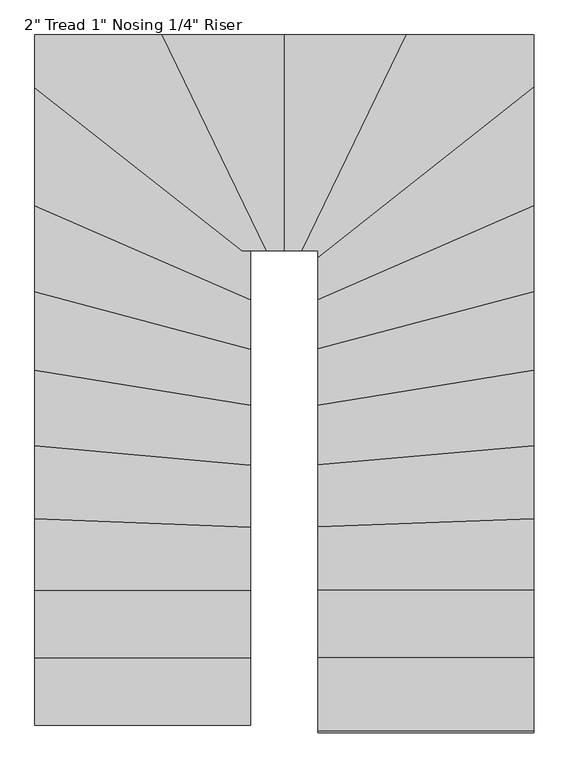
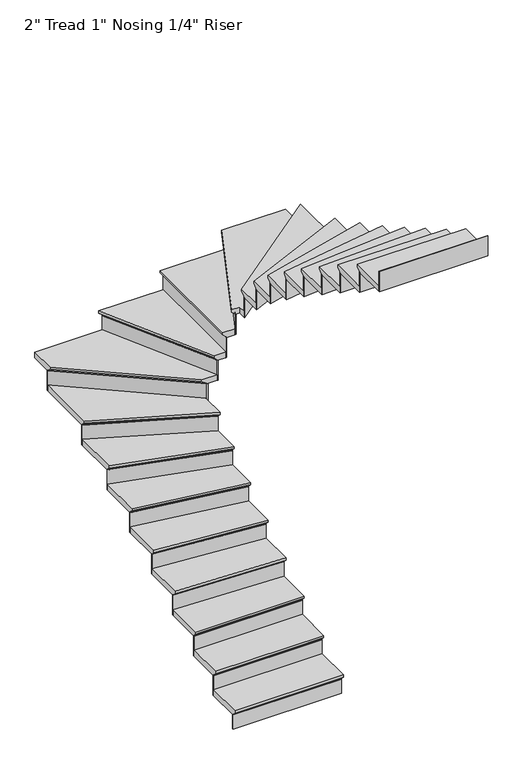
"""IFC4 building model written with IfcOpenShell, lengths in millimetres: stair flight geometry."""

from ifc_helpers import new_model, si_unit, origin, place, context, project, spatial, faceted_brep, source, transform, mapped, element, save


def stair_flight_c7d98fdd(model_context):
    return source(origin(), model_context, "Body", "Brep", [
        faceted_brep([(-5047.1987704, -4554.2130548, 47703.9214286), (-5047.1987704, -4554.2130548, 47722.9714286), (-5940.8822214, -4554.2130548, 47722.9714286), (-5940.8822214, -4554.2130548, 47703.9214286), (-5047.1987704, -4528.8130548, 47678.5214286), (-5940.8822214, -4528.8130548, 47678.5214286), (-5047.1987704, -4249.4130548, 47722.9714286), (-5940.8822214, -4249.4130548, 47722.9714286), (-5940.8822214, -4528.8130548, 47672.1714286), (-5940.8822214, -4249.4130548, 47672.1714286), (-5047.1987704, -4249.4130548, 47672.1714286), (-5047.1987704, -4528.8130548, 47672.1714286)], [[[0, 1, 2, 3]], [[4, 0, 3, 5]], [[2, 1, 6, 7]], [[8, 9, 10, 11]], [[2, 7, 9, 8, 5, 3]], [[8, 11, 4, 5]], [[6, 1, 0, 4, 11, 10]], [[7, 6, 10, 9]]]),
        faceted_brep([(-5047.1987704, -4528.8130548, 47672.1714286), (-5047.1987704, -4528.8130548, 47548.8), (-5047.1987704, -4522.4630548, 47548.8), (-5047.1987704, -4522.4630548, 47672.1714286), (-5940.8822214, -4528.8130548, 47672.1714286), (-5940.8822214, -4522.4630548, 47672.1714286), (-5940.8822214, -4522.4630548, 47548.8), (-5940.8822214, -4528.8130548, 47548.8)], [[[0, 1, 2, 3]], [[4, 5, 6, 7]], [[1, 0, 4, 7]], [[2, 1, 7, 6]], [[3, 2, 6, 5]], [[0, 3, 5, 4]]]),
        faceted_brep([(-5047.1987704, -4249.4130548, 47846.3428571), (-5047.1987704, -4249.4130548, 47672.1714286), (-5047.1987704, -4243.0630548, 47672.1714286), (-5047.1987704, -4243.0630548, 47846.3428571), (-5940.8822214, -4249.4130548, 47846.3428571), (-5940.8822214, -4243.0630548, 47846.3428571), (-5940.8822214, -4243.0630548, 47672.1714286), (-5940.8822214, -4249.4130548, 47672.1714286)], [[[0, 1, 2, 3]], [[4, 5, 6, 7]], [[1, 0, 4, 7]], [[2, 1, 7, 6]], [[3, 2, 6, 5]], [[0, 3, 5, 4]]]),
        faceted_brep([(-5940.8822214, -4274.8130548, 47897.1428571), (-5047.1987704, -4274.8130548, 47897.1428571), (-5047.1987704, -3970.0130548, 47897.1428571), (-5940.8822214, -3970.0130548, 47897.1428571), (-5940.8822214, -4249.4130548, 47846.3428571), (-5940.8822214, -3970.0130548, 47846.3428571), (-5047.1987704, -3970.0130548, 47846.3428571), (-5047.1987704, -4249.4130548, 47846.3428571), (-5940.8822214, -4249.4130548, 47852.6928571), (-5940.8822214, -4274.8130548, 47878.0928571), (-5047.1987704, -4249.4130548, 47852.6928571), (-5047.1987704, -4274.8130548, 47878.0928571)], [[[0, 1, 2, 3]], [[4, 5, 6, 7]], [[0, 3, 5, 4, 8, 9]], [[4, 7, 10, 8]], [[2, 1, 11, 10, 7, 6]], [[3, 2, 6, 5]], [[11, 1, 0, 9]], [[10, 11, 9, 8]]]),
        faceted_brep([(-5047.1987704, -3970.0130548, 48020.5142857), (-5047.1987704, -3970.0130548, 47846.3428571), (-5047.1987704, -3963.6630548, 47846.3428571), (-5047.1987704, -3963.6630548, 48020.5142857), (-5940.8822214, -3970.0130548, 48020.5142857), (-5940.8822214, -3963.6630548, 48020.5142857), (-5940.8822214, -3963.6630548, 47846.3428571), (-5940.8822214, -3970.0130548, 47846.3428571)], [[[0, 1, 2, 3]], [[4, 5, 6, 7]], [[1, 0, 4, 7]], [[2, 1, 7, 6]], [[3, 2, 6, 5]], [[0, 3, 5, 4]]]),
        faceted_brep([(-5940.8822214, -3995.4130548, 48071.3142857), (-5047.1987704, -3995.4130548, 48071.3142857), (-5047.1987704, -3707.9036879, 48071.3142857), (-5940.8822214, -3673.2843203, 48071.3142857), (-5940.8822214, -3970.0130548, 48020.5142857), (-5940.8822214, -3673.2843203, 48020.5142857), (-5047.1987704, -3707.9036879, 48020.5142857), (-5047.1987704, -3970.0130548, 48020.5142857), (-5940.8822214, -3970.0130548, 48026.8642857), (-5940.8822214, -3995.4130548, 48052.2642857), (-5047.1987704, -3970.0130548, 48026.8642857), (-5047.1987704, -3995.4130548, 48052.2642857)], [[[0, 1, 2, 3]], [[4, 5, 6, 7]], [[0, 3, 5, 4, 8, 9]], [[4, 7, 10, 8]], [[2, 1, 11, 10, 7, 6]], [[3, 2, 6, 5]], [[11, 1, 0, 9]], [[10, 11, 9, 8]]]),
        faceted_brep([(-5047.1987704, -3707.9036879, 48194.6857143), (-5047.1987704, -3707.9036879, 48020.5142857), (-5047.1987704, -3701.5489252, 48020.5142857), (-5047.1987704, -3701.5489252, 48194.6857143), (-5940.8822214, -3673.2843203, 48194.6857143), (-5940.8822214, -3666.9295576, 48194.6857143), (-5940.8822214, -3666.9295576, 48020.5142857), (-5940.8822214, -3673.2843203, 48020.5142857)], [[[0, 1, 2, 3]], [[4, 5, 6, 7]], [[1, 0, 4, 7]], [[2, 1, 7, 6]], [[3, 2, 6, 5]], [[0, 3, 5, 4]]]),
        faceted_brep([(-5940.8822214, -3698.703371, 48245.4857143), (-5047.1987704, -3733.3227386, 48245.4857143), (-5047.1987704, -3451.3234819, 48245.4857143), (-5940.8822214, -3370.89733, 48245.4857143), (-5940.8822214, -3673.2843203, 48194.6857143), (-5940.8822214, -3370.89733, 48194.6857143), (-5047.1987704, -3451.3234819, 48194.6857143), (-5047.1987704, -3707.9036879, 48194.6857143), (-5940.8822214, -3673.2843203, 48201.0357143), (-5940.8822214, -3698.703371, 48226.4357143), (-5047.1987704, -3707.9036879, 48201.0357143), (-5047.1987704, -3733.3227386, 48226.4357143)], [[[0, 1, 2, 3]], [[4, 5, 6, 7]], [[0, 3, 5, 4, 8, 9]], [[4, 7, 10, 8]], [[2, 1, 11, 10, 7, 6]], [[3, 2, 6, 5]], [[11, 1, 0, 9]], [[10, 11, 9, 8]]]),
        faceted_brep([(-5047.1987704, -3451.3234819, 48368.8571429), (-5047.1987704, -3451.3234819, 48194.6857143), (-5047.1987704, -3444.9478197, 48194.6857143), (-5047.1987704, -3444.9478197, 48368.8571429), (-5940.8822214, -3370.89733, 48368.8571429), (-5940.8822214, -3364.5216678, 48368.8571429), (-5940.8822214, -3364.5216678, 48194.6857143), (-5940.8822214, -3370.89733, 48194.6857143)], [[[0, 1, 2, 3]], [[4, 5, 6, 7]], [[1, 0, 4, 7]], [[2, 1, 7, 6]], [[3, 2, 6, 5]], [[0, 3, 5, 4]]]),
        faceted_brep([(-5940.8822214, -3396.3999789, 48419.6571429), (-5047.1987704, -3476.8261308, 48419.6571429), (-5047.1987704, -3203.4301079, 48419.6571429), (-5940.8822214, -3059.5417727, 48419.6571429), (-5940.8822214, -3370.89733, 48368.8571429), (-5940.8822214, -3059.5417727, 48368.8571429), (-5047.1987704, -3203.4301079, 48368.8571429), (-5047.1987704, -3451.3234819, 48368.8571429), (-5940.8822214, -3370.89733, 48375.2071429), (-5940.8822214, -3396.3999789, 48400.6071429), (-5047.1987704, -3451.3234819, 48375.2071429), (-5047.1987704, -3476.8261308, 48400.6071429)], [[[0, 1, 2, 3]], [[4, 5, 6, 7]], [[0, 3, 5, 4, 8, 9]], [[4, 7, 10, 8]], [[2, 1, 11, 10, 7, 6]], [[3, 2, 6, 5]], [[11, 1, 0, 9]], [[10, 11, 9, 8]]]),
        faceted_brep([(-5047.1987704, -3203.4301079, 48543.0285714), (-5047.1987704, -3203.4301079, 48368.8571429), (-5047.1987704, -3196.9983292, 48368.8571429), (-5047.1987704, -3196.9983292, 48543.0285714), (-5940.8822214, -3059.5417727, 48543.0285714), (-5940.8822214, -3053.109994, 48543.0285714), (-5940.8822214, -3053.109994, 48368.8571429), (-5940.8822214, -3059.5417727, 48368.8571429)], [[[0, 1, 2, 3]], [[4, 5, 6, 7]], [[1, 0, 4, 7]], [[2, 1, 7, 6]], [[3, 2, 6, 5]], [[0, 3, 5, 4]]]),
        faceted_brep([(-5940.8822214, -3085.2688872, 48593.8285714), (-5047.1987704, -3229.1572224, 48593.8285714), (-5047.1987704, -2970.3553609, 48593.8285714), (-5940.8822214, -2732.7052783, 48593.8285714), (-5940.8822214, -3059.5417727, 48543.0285714), (-5940.8822214, -2732.7052783, 48543.0285714), (-5047.1987704, -2970.3553609, 48543.0285714), (-5047.1987704, -3203.4301079, 48543.0285714), (-5940.8822214, -3059.5417727, 48549.3785714), (-5940.8822214, -3085.2688872, 48574.7785714), (-5047.1987704, -3203.4301079, 48549.3785714), (-5047.1987704, -3229.1572224, 48574.7785714)], [[[0, 1, 2, 3]], [[4, 5, 6, 7]], [[0, 3, 5, 4, 8, 9]], [[4, 7, 10, 8]], [[2, 1, 11, 10, 7, 6]], [[3, 2, 6, 5]], [[11, 1, 0, 9]], [[10, 11, 9, 8]]]),
        faceted_brep([(-5047.1987704, -2970.3553609, 48717.2), (-5047.1987704, -2970.3553609, 48543.0285714), (-5047.1987704, -2963.7846771, 48543.0285714), (-5047.1987704, -2963.7846771, 48717.2), (-5940.8822214, -2732.7052783, 48717.2), (-5940.8822214, -2726.1345945, 48717.2), (-5940.8822214, -2726.1345945, 48543.0285714), (-5940.8822214, -2732.7052783, 48543.0285714)], [[[0, 1, 2, 3]], [[4, 5, 6, 7]], [[1, 0, 4, 7]], [[2, 1, 7, 6]], [[3, 2, 6, 5]], [[0, 3, 5, 4]]]),
        faceted_brep([(-5940.8822214, -2758.9880136, 48768.0), (-5047.1987704, -2996.6380961, 48768.0), (-5047.1987704, -2765.8050203, 48768.0), (-5940.8822214, -2375.5896532, 48768.0), (-5940.8822214, -2732.7052783, 48717.2), (-5940.8822214, -2375.5896532, 48717.2), (-5047.1987704, -2765.8050203, 48717.2), (-5047.1987704, -2970.3553609, 48717.2), (-5940.8822214, -2732.7052783, 48723.55), (-5940.8822214, -2758.9880136, 48748.95), (-5047.1987704, -2970.3553609, 48723.55), (-5047.1987704, -2996.6380961, 48748.95)], [[[0, 1, 2, 3]], [[4, 5, 6, 7]], [[0, 3, 5, 4, 8, 9]], [[4, 7, 10, 8]], [[2, 1, 11, 10, 7, 6]], [[3, 2, 6, 5]], [[11, 1, 0, 9]], [[10, 11, 9, 8]]]),
        faceted_brep([(-5047.1987704, -2765.8050203, 48891.3714286), (-5047.1987704, -2765.8050203, 48717.2), (-5047.1987704, -2758.8760908, 48717.2), (-5047.1987704, -2758.8760908, 48891.3714286), (-5940.8822214, -2375.5896532, 48891.3714286), (-5940.8822214, -2368.6607237, 48891.3714286), (-5940.8822214, -2368.6607237, 48717.2), (-5940.8822214, -2375.5896532, 48717.2)], [[[0, 1, 2, 3]], [[4, 5, 6, 7]], [[1, 0, 4, 7]], [[2, 1, 7, 6]], [[3, 2, 6, 5]], [[0, 3, 5, 4]]]),
        faceted_brep([(-5940.8822214, -2403.3053713, 48942.1714286), (-5047.1987704, -2793.5207384, 48942.1714286), (-5047.1987704, -2590.8424524, 48942.1714286), (-5040.8038639, -2590.8424524, 48942.1714286), (-5940.8822214, -1882.1944717, 48942.1714286), (-5940.8822214, -2375.5896532, 48891.3714286), (-5940.8822214, -1882.1944717, 48891.3714286), (-5040.8038639, -2590.8424524, 48891.3714286), (-5047.1987704, -2590.8424524, 48891.3714286), (-5047.1987704, -2765.8050203, 48891.3714286), (-5940.8822214, -2375.5896532, 48897.7214286), (-5940.8822214, -2403.3053713, 48923.1214286), (-5047.1987704, -2765.8050203, 48897.7214286), (-5047.1987704, -2793.5207384, 48923.1214286)], [[[0, 1, 2, 3, 4]], [[5, 6, 7, 8, 9]], [[0, 4, 6, 5, 10, 11]], [[5, 9, 12, 10]], [[2, 1, 13, 12, 9, 8]], [[4, 3, 7, 6]], [[13, 1, 0, 11]], [[12, 13, 11, 10]], [[3, 2, 8, 7]]]),
        faceted_brep([(-5040.8038639, -2590.8424524, 49065.5428571), (-5040.8038639, -2590.8424524, 48891.3714286), (-5030.5387554, -2590.8424524, 48891.3714286), (-5030.5387554, -2590.8424524, 49065.5428571), (-5940.8822214, -1882.1944717, 49065.5428571), (-5940.8822214, -1874.1125661, 49065.5428571), (-5940.8822214, -1874.1125661, 48891.3714286), (-5940.8822214, -1882.1944717, 48891.3714286)], [[[0, 1, 2, 3]], [[4, 5, 6, 7]], [[1, 0, 4, 7]], [[2, 1, 7, 6]], [[3, 2, 6, 5]], [[0, 3, 5, 4]]]),
        faceted_brep([(-5384.6489457, -1697.1590014, 49116.3428571), (-5940.8822214, -1697.1590014, 49116.3428571), (-5940.8822214, -1914.5220945, 49116.3428571), (-5081.8642978, -2590.8424524, 49116.3428571), (-4952.3566185, -2590.8424524, 49116.3428571), (-5940.8822214, -1697.1590014, 49065.5428571), (-5384.6489457, -1697.1590014, 49065.5428571), (-4952.3566185, -2590.8424524, 49065.5428571), (-5040.8038639, -2590.8424524, 49065.5428571), (-5940.8822214, -1882.1944717, 49065.5428571), (-5940.8822214, -1882.1944717, 49071.8928571), (-5940.8822214, -1914.5220945, 49097.2928571), (-5040.8038639, -2590.8424524, 49071.8928571), (-5081.8642978, -2590.8424524, 49097.2928571)], [[[0, 1, 2, 3, 4]], [[5, 6, 7, 8, 9]], [[1, 0, 6, 5]], [[2, 1, 5, 9, 10, 11]], [[9, 8, 12, 10]], [[4, 3, 13, 12, 8, 7]], [[0, 4, 7, 6]], [[13, 3, 2, 11]], [[12, 13, 11, 10]]]),
        faceted_brep([(-4952.3566185, -2590.8424524, 49239.7142857), (-4952.3566185, -2590.8424524, 49065.5428571), (-4945.3027294, -2590.8424524, 49065.5428571), (-4945.3027294, -2590.8424524, 49239.7142857), (-5384.6489457, -1697.1590014, 49239.7142857), (-5377.5950566, -1697.1590014, 49239.7142857), (-5377.5950566, -1697.1590014, 49065.5428571), (-5384.6489457, -1697.1590014, 49065.5428571)], [[[0, 1, 2, 3]], [[4, 5, 6, 7]], [[1, 0, 4, 7]], [[2, 1, 7, 6]], [[3, 2, 6, 5]], [[0, 3, 5, 4]]]),
        faceted_brep([(-5412.8645022, -1697.1590014, 49290.5142857), (-4980.5721749, -2590.8424524, 49290.5142857), (-4882.0987704, -2590.8424524, 49290.5142857), (-4882.0987706, -1697.1590014, 49290.5142857), (-5384.6489457, -1697.1590014, 49239.7142857), (-4882.0987706, -1697.1590014, 49239.7142857), (-4882.0987704, -2590.8424524, 49239.7142857), (-4952.3566185, -2590.8424524, 49239.7142857), (-5384.6489457, -1697.1590014, 49246.0642857), (-5412.8645022, -1697.1590014, 49271.4642857), (-4952.3566185, -2590.8424524, 49246.0642857), (-4980.5721749, -2590.8424524, 49271.4642857)], [[[0, 1, 2, 3]], [[4, 5, 6, 7]], [[0, 3, 5, 4, 8, 9]], [[4, 7, 10, 8]], [[3, 2, 6, 5]], [[11, 1, 0, 9]], [[10, 11, 9, 8]], [[2, 1, 11, 10, 7, 6]]]),
        faceted_brep([(-4882.0987704, -2590.8424524, 49413.8857143), (-4882.0987704, -2590.8424524, 49239.7142857), (-4875.7487704, -2590.8424524, 49239.7142857), (-4875.7487704, -2590.8424524, 49413.8857143), (-4882.0987706, -1697.1590014, 49413.8857143), (-4875.7487706, -1697.1590014, 49413.8857143), (-4875.7487706, -1697.1590014, 49239.7142857), (-4882.0987706, -1697.1590014, 49239.7142857)], [[[0, 1, 2, 3]], [[4, 5, 6, 7]], [[1, 0, 4, 7]], [[2, 1, 7, 6]], [[3, 2, 6, 5]], [[0, 3, 5, 4]]]),
        faceted_brep([(-4907.4987706, -1697.1590014, 49464.6857143), (-4907.4987704, -2590.8424524, 49464.6857143), (-4806.2098095, -2590.8424524, 49464.6857143), (-4373.9174828, -1697.1590014, 49464.6857143), (-4882.0987706, -1697.1590014, 49413.8857143), (-4373.9174828, -1697.1590014, 49413.8857143), (-4806.2098095, -2590.8424524, 49413.8857143), (-4882.0987704, -2590.8424524, 49413.8857143), (-4882.0987706, -1697.1590014, 49420.2357143), (-4907.4987706, -1697.1590014, 49445.6357143), (-4882.0987704, -2590.8424524, 49420.2357143), (-4907.4987704, -2590.8424524, 49445.6357143)], [[[0, 1, 2, 3]], [[4, 5, 6, 7]], [[0, 3, 5, 4, 8, 9]], [[4, 7, 10, 8]], [[2, 1, 11, 10, 7, 6]], [[3, 2, 6, 5]], [[11, 1, 0, 9]], [[10, 11, 9, 8]]]),
        faceted_brep([(-4806.2098095, -2590.8424524, 49588.0571429), (-4806.2098095, -2590.8424524, 49413.8857143), (-4799.1559204, -2590.8424524, 49413.8857143), (-4799.1559204, -2590.8424524, 49588.0571429), (-4373.9174828, -1697.1590014, 49588.0571429), (-4366.8635937, -1697.1590014, 49588.0571429), (-4366.8635937, -1697.1590014, 49413.8857143), (-4373.9174828, -1697.1590014, 49413.8857143)], [[[0, 1, 2, 3]], [[4, 5, 6, 7]], [[1, 0, 4, 7]], [[2, 1, 7, 6]], [[3, 2, 6, 5]], [[0, 3, 5, 4]]]),
        faceted_brep([(-3874.1153195, -1946.8497166, 49638.8571429), (-3874.1153195, -1697.1590014, 49638.8571429), (-4402.1330392, -1697.1590014, 49638.8571429), (-4834.4253659, -2590.8424524, 49638.8571429), (-4767.7987704, -2590.8424524, 49638.8571429), (-4767.7987704, -2650.4628721, 49638.8571429), (-3874.1153195, -1697.1590014, 49588.0571429), (-3874.1153195, -1946.8497166, 49588.0571429), (-4767.7987704, -2650.4628721, 49588.0571429), (-4767.7987704, -2590.8424524, 49588.0571429), (-4806.2098095, -2590.8424524, 49588.0571429), (-4373.9174828, -1697.1590014, 49588.0571429), (-4806.2098095, -2590.8424524, 49594.4071429), (-4373.9174828, -1697.1590014, 49594.4071429), (-4834.4253659, -2590.8424524, 49619.8071429), (-4402.1330392, -1697.1590014, 49619.8071429)], [[[0, 1, 2, 3, 4, 5]], [[6, 7, 8, 9, 10, 11]], [[1, 0, 7, 6]], [[11, 10, 12, 13]], [[4, 3, 14, 12, 10, 9]], [[5, 4, 9, 8]], [[0, 5, 8, 7]], [[14, 3, 2, 15]], [[12, 14, 15, 13]], [[2, 1, 6, 11, 13, 15]]]),
        faceted_brep([(-4767.7987704, -2650.4628721, 49762.2285714), (-4767.7987704, -2650.4628721, 49588.0571429), (-4767.7987704, -2658.5447778, 49588.0571429), (-4767.7987704, -2658.5447778, 49762.2285714), (-3874.1153195, -1946.8497166, 49762.2285714), (-3874.1153195, -1954.9316222, 49762.2285714), (-3874.1153195, -1954.9316222, 49588.0571429), (-3874.1153195, -1946.8497166, 49588.0571429)], [[[0, 1, 2, 3]], [[4, 5, 6, 7]], [[1, 0, 4, 7]], [[2, 1, 7, 6]], [[3, 2, 6, 5]], [[0, 3, 5, 4]]]),
        faceted_brep([(-3874.1153195, -1914.5220938, 49813.0285714), (-4767.7987704, -2618.1352494, 49813.0285714), (-4767.7987704, -2821.2364563, 49813.0285714), (-3874.1153195, -2431.0210889, 49813.0285714), (-3874.1153195, -1946.8497166, 49762.2285714), (-3874.1153195, -2431.0210889, 49762.2285714), (-4767.7987704, -2821.2364563, 49762.2285714), (-4767.7987704, -2650.4628721, 49762.2285714), (-3874.1153195, -1946.8497166, 49768.5785714), (-3874.1153195, -1914.5220938, 49793.9785714), (-4767.7987704, -2650.4628721, 49768.5785714), (-4767.7987704, -2618.1352494, 49793.9785714)], [[[0, 1, 2, 3]], [[4, 5, 6, 7]], [[0, 3, 5, 4, 8, 9]], [[4, 7, 10, 8]], [[2, 1, 11, 10, 7, 6]], [[3, 2, 6, 5]], [[11, 1, 0, 9]], [[10, 11, 9, 8]]]),
        faceted_brep([(-4767.7987704, -2821.2364563, 49936.4), (-4767.7987704, -2821.2364563, 49762.2285714), (-4767.7987704, -2828.1653858, 49762.2285714), (-4767.7987704, -2828.1653858, 49936.4), (-3874.1153195, -2431.0210889, 49936.4), (-3874.1153195, -2437.9500185, 49936.4), (-3874.1153195, -2437.9500185, 49762.2285714), (-3874.1153195, -2431.0210889, 49762.2285714)], [[[0, 1, 2, 3]], [[4, 5, 6, 7]], [[1, 0, 4, 7]], [[2, 1, 7, 6]], [[3, 2, 6, 5]], [[0, 3, 5, 4]]]),
        faceted_brep([(-3874.1153195, -2403.3053709, 49987.2), (-4767.7987704, -2793.5207382, 49987.2), (-4767.7987704, -3022.9208311, 49987.2), (-3874.1153195, -2785.2707484, 49987.2), (-3874.1153195, -2431.0210889, 49936.4), (-3874.1153195, -2785.2707484, 49936.4), (-4767.7987704, -3022.9208311, 49936.4), (-4767.7987704, -2821.2364563, 49936.4), (-3874.1153195, -2431.0210889, 49942.75), (-3874.1153195, -2403.3053709, 49968.15), (-4767.7987704, -2821.2364563, 49942.75), (-4767.7987704, -2793.5207382, 49968.15)], [[[0, 1, 2, 3]], [[4, 5, 6, 7]], [[0, 3, 5, 4, 8, 9]], [[4, 7, 10, 8]], [[2, 1, 11, 10, 7, 6]], [[3, 2, 6, 5]], [[11, 1, 0, 9]], [[10, 11, 9, 8]]]),
        faceted_brep([(-4767.7987704, -3022.9208311, 50110.5714286), (-4767.7987704, -3022.9208311, 49936.4), (-4767.7987704, -3029.4915149, 49936.4), (-4767.7987704, -3029.4915149, 50110.5714286), (-3874.1153195, -2785.2707484, 50110.5714286), (-3874.1153195, -2791.8414322, 50110.5714286), (-3874.1153195, -2791.8414322, 49936.4), (-3874.1153195, -2785.2707484, 49936.4)], [[[0, 1, 2, 3]], [[4, 5, 6, 7]], [[1, 0, 4, 7]], [[2, 1, 7, 6]], [[3, 2, 6, 5]], [[0, 3, 5, 4]]]),
        faceted_brep([(-3874.1153195, -2758.9880132, 50161.3714286), (-4767.7987704, -2996.6380959, 50161.3714286), (-4767.7987704, -3254.8843368, 50161.3714286), (-3874.1153195, -3110.9960015, 50161.3714286), (-3874.1153195, -2785.2707484, 50110.5714286), (-3874.1153195, -3110.9960015, 50110.5714286), (-4767.7987704, -3254.8843368, 50110.5714286), (-4767.7987704, -3022.9208311, 50110.5714286), (-3874.1153195, -2785.2707484, 50116.9214286), (-3874.1153195, -2758.9880132, 50142.3214286), (-4767.7987704, -3022.9208311, 50116.9214286), (-4767.7987704, -2996.6380959, 50142.3214286)], [[[0, 1, 2, 3]], [[4, 5, 6, 7]], [[0, 3, 5, 4, 8, 9]], [[4, 7, 10, 8]], [[2, 1, 11, 10, 7, 6]], [[3, 2, 6, 5]], [[11, 1, 0, 9]], [[10, 11, 9, 8]]]),
        faceted_brep([(-4767.7987704, -3254.8843368, 50284.7428571), (-4767.7987704, -3254.8843368, 50110.5714286), (-4767.7987704, -3261.3161154, 50110.5714286), (-4767.7987704, -3261.3161154, 50284.7428571), (-3874.1153195, -3110.9960015, 50284.7428571), (-3874.1153195, -3117.4277801, 50284.7428571), (-3874.1153195, -3117.4277801, 50110.5714286), (-3874.1153195, -3110.9960015, 50110.5714286)], [[[0, 1, 2, 3]], [[4, 5, 6, 7]], [[1, 0, 4, 7]], [[2, 1, 7, 6]], [[3, 2, 6, 5]], [[0, 3, 5, 4]]]),
        faceted_brep([(-3874.1153195, -3085.2688869, 50335.5428571), (-4767.7987704, -3229.1572222, 50335.5428571), (-4767.7987704, -3502.3287795, 50335.5428571), (-3874.1153195, -3421.9026274, 50335.5428571), (-3874.1153195, -3110.9960015, 50284.7428571), (-3874.1153195, -3421.9026274, 50284.7428571), (-4767.7987704, -3502.3287795, 50284.7428571), (-4767.7987704, -3254.8843368, 50284.7428571), (-3874.1153195, -3110.9960015, 50291.0928571), (-3874.1153195, -3085.2688869, 50316.4928571), (-4767.7987704, -3254.8843368, 50291.0928571), (-4767.7987704, -3229.1572222, 50316.4928571)], [[[0, 1, 2, 3]], [[4, 5, 6, 7]], [[0, 3, 5, 4, 8, 9]], [[4, 7, 10, 8]], [[2, 1, 11, 10, 7, 6]], [[3, 2, 6, 5]], [[11, 1, 0, 9]], [[10, 11, 9, 8]]]),
        faceted_brep([(-4767.7987704, -3502.3287795, 50458.9142857), (-4767.7987704, -3502.3287795, 50284.7428571), (-4767.7987704, -3508.7044417, 50284.7428571), (-4767.7987704, -3508.7044417, 50458.9142857), (-3874.1153195, -3421.9026274, 50458.9142857), (-3874.1153195, -3428.2782897, 50458.9142857), (-3874.1153195, -3428.2782897, 50284.7428571), (-3874.1153195, -3421.9026274, 50284.7428571)], [[[0, 1, 2, 3]], [[4, 5, 6, 7]], [[1, 0, 4, 7]], [[2, 1, 7, 6]], [[3, 2, 6, 5]], [[0, 3, 5, 4]]]),
        faceted_brep([(-3874.1153195, -3396.3999786, 50509.7142857), (-4767.7987704, -3476.8261306, 50509.7142857), (-4767.7987704, -3758.7417891, 50509.7142857), (-3874.1153195, -3724.1224215, 50509.7142857), (-3874.1153195, -3421.9026274, 50458.9142857), (-3874.1153195, -3724.1224215, 50458.9142857), (-4767.7987704, -3758.7417891, 50458.9142857), (-4767.7987704, -3502.3287795, 50458.9142857), (-3874.1153195, -3421.9026274, 50465.2642857), (-3874.1153195, -3396.3999786, 50490.6642857), (-4767.7987704, -3502.3287795, 50465.2642857), (-4767.7987704, -3476.8261306, 50490.6642857)], [[[0, 1, 2, 3]], [[4, 5, 6, 7]], [[0, 3, 5, 4, 8, 9]], [[4, 7, 10, 8]], [[2, 1, 11, 10, 7, 6]], [[3, 2, 6, 5]], [[11, 1, 0, 9]], [[10, 11, 9, 8]]]),
        faceted_brep([(-4767.7987704, -3758.7417891, 50633.0857143), (-4767.7987704, -3758.7417891, 50458.9142857), (-4767.7987704, -3765.0965518, 50458.9142857), (-4767.7987704, -3765.0965518, 50633.0857143), (-3874.1153195, -3724.1224215, 50633.0857143), (-3874.1153195, -3730.4771842, 50633.0857143), (-3874.1153195, -3730.4771842, 50458.9142857), (-3874.1153195, -3724.1224215, 50458.9142857)], [[[0, 1, 2, 3]], [[4, 5, 6, 7]], [[1, 0, 4, 7]], [[2, 1, 7, 6]], [[3, 2, 6, 5]], [[0, 3, 5, 4]]]),
        faceted_brep([(-3874.1153195, -3698.7033708, 50683.8857143), (-4767.7987704, -3733.3227384, 50683.8857143), (-4767.7987704, -4020.8130546, 50683.8857143), (-3874.1153195, -4020.8130546, 50683.8857143), (-3874.1153195, -3724.1224215, 50633.0857143), (-3874.1153195, -4020.8130546, 50633.0857143), (-4767.7987704, -4020.8130546, 50633.0857143), (-4767.7987704, -3758.7417891, 50633.0857143), (-3874.1153195, -3724.1224215, 50639.4357143), (-3874.1153195, -3698.7033708, 50664.8357143), (-4767.7987704, -3758.7417891, 50639.4357143), (-4767.7987704, -3733.3227384, 50664.8357143)], [[[0, 1, 2, 3]], [[4, 5, 6, 7]], [[0, 3, 5, 4, 8, 9]], [[4, 7, 10, 8]], [[2, 1, 11, 10, 7, 6]], [[3, 2, 6, 5]], [[11, 1, 0, 9]], [[10, 11, 9, 8]]]),
        faceted_brep([(-4767.7987704, -4020.8130546, 50807.2571429), (-4767.7987704, -4020.8130546, 50633.0857143), (-4767.7987704, -4027.1630546, 50633.0857143), (-4767.7987704, -4027.1630546, 50807.2571429), (-3874.1153195, -4020.8130546, 50807.2571429), (-3874.1153195, -4027.1630546, 50807.2571429), (-3874.1153195, -4027.1630546, 50633.0857143), (-3874.1153195, -4020.8130546, 50633.0857143)], [[[0, 1, 2, 3]], [[4, 5, 6, 7]], [[1, 0, 4, 7]], [[2, 1, 7, 6]], [[3, 2, 6, 5]], [[0, 3, 5, 4]]]),
        faceted_brep([(-3874.1153195, -3995.4130546, 50858.0571429), (-4767.7987704, -3995.4130546, 50858.0571429), (-4767.7987704, -4300.2130546, 50858.0571429), (-3874.1153195, -4300.2130546, 50858.0571429), (-3874.1153195, -4020.8130546, 50807.2571429), (-3874.1153195, -4300.2130546, 50807.2571429), (-4767.7987704, -4300.2130546, 50807.2571429), (-4767.7987704, -4020.8130546, 50807.2571429), (-3874.1153195, -4020.8130546, 50813.6071429), (-3874.1153195, -3995.4130546, 50839.0071429), (-4767.7987704, -4020.8130546, 50813.6071429), (-4767.7987704, -3995.4130546, 50839.0071429)], [[[0, 1, 2, 3]], [[4, 5, 6, 7]], [[0, 3, 5, 4, 8, 9]], [[4, 7, 10, 8]], [[2, 1, 11, 10, 7, 6]], [[3, 2, 6, 5]], [[11, 1, 0, 9]], [[10, 11, 9, 8]]]),
        faceted_brep([(-4767.7987704, -4300.2130546, 50981.4285714), (-4767.7987704, -4300.2130546, 50807.2571429), (-4767.7987704, -4306.5630546, 50807.2571429), (-4767.7987704, -4306.5630546, 50981.4285714), (-3874.1153195, -4300.2130546, 50981.4285714), (-3874.1153195, -4306.5630546, 50981.4285714), (-3874.1153195, -4306.5630546, 50807.2571429), (-3874.1153195, -4300.2130546, 50807.2571429)], [[[0, 1, 2, 3]], [[4, 5, 6, 7]], [[1, 0, 4, 7]], [[2, 1, 7, 6]], [[3, 2, 6, 5]], [[0, 3, 5, 4]]]),
        faceted_brep([(-4767.7987704, -4579.6130546, 51155.6), (-4767.7987704, -4579.6130546, 50981.4285714), (-4767.7987704, -4585.9630546, 50981.4285714), (-4767.7987704, -4585.9630546, 51155.6), (-3874.1153195, -4579.6130546, 51155.6), (-3874.1153195, -4585.9630546, 51155.6), (-3874.1153195, -4585.9630546, 50981.4285714), (-3874.1153195, -4579.6130546, 50981.4285714)], [[[0, 1, 2, 3]], [[4, 5, 6, 7]], [[1, 0, 4, 7]], [[2, 1, 7, 6]], [[3, 2, 6, 5]], [[0, 3, 5, 4]]]),
        faceted_brep([(-3874.1153195, -4274.8130546, 51032.2285714), (-4767.7987704, -4274.8130546, 51032.2285714), (-4767.7987704, -4579.6130546, 51032.2285714), (-3874.1153195, -4579.6130546, 51032.2285714), (-3874.1153195, -4300.2130546, 50981.4285714), (-3874.1153195, -4579.6130546, 50981.4285714), (-4767.7987704, -4579.6130546, 50981.4285714), (-4767.7987704, -4300.2130546, 50981.4285714), (-3874.1153195, -4300.2130546, 50987.7785714), (-3874.1153195, -4274.8130546, 51013.1785714), (-4767.7987704, -4300.2130546, 50987.7785714), (-4767.7987704, -4274.8130546, 51013.1785714)], [[[0, 1, 2, 3]], [[4, 5, 6, 7]], [[0, 3, 5, 4, 8, 9]], [[4, 7, 10, 8]], [[2, 1, 11, 10, 7, 6]], [[3, 2, 6, 5]], [[11, 1, 0, 9]], [[10, 11, 9, 8]]]),
    ])


if __name__ == "__main__":
    model = new_model("IFC4")
    model_context = context("Model", 3, world=origin())
    ifc_project = project(units=[si_unit("LENGTHUNIT", "METRE", prefix="MILLI")], contexts=[model_context])
    site = spatial("IfcSite", under=ifc_project)
    building = spatial("IfcBuilding", under=site)
    placement = place(None, origin())
    stair_flight_shape = stair_flight_c7d98fdd(model_context)
    element("IfcStairFlight", 1, ObjectType="2\" Tread 1\" Nosing 1/4\" Riser", at=placement, inside=building, context=model_context, shape_type="MappedRepresentation", body=[
        mapped(stair_flight_shape, transform((0.0, 0.0, 0.0), x_axis=(1.0, 0.0, 0.0), y_axis=(0.0, 1.0, 0.0), z_axis=(0.0, 0.0, 1.0))),
    ])
    save(model, "model.ifc")

# Revit data of these elements
# Element 1 (IfcStairFlight, "2\" Tread 1\" Nosing 1/4\" Riser")
#   Materials on its faces: "Tile, Porcelain, 4in"
# Materials
#   "Tile, Porcelain, 4in": class "Generic", colour RGB 89 87 158, transparency 0, Description = "Porcelain tile, 4\", white", Cost = 0
